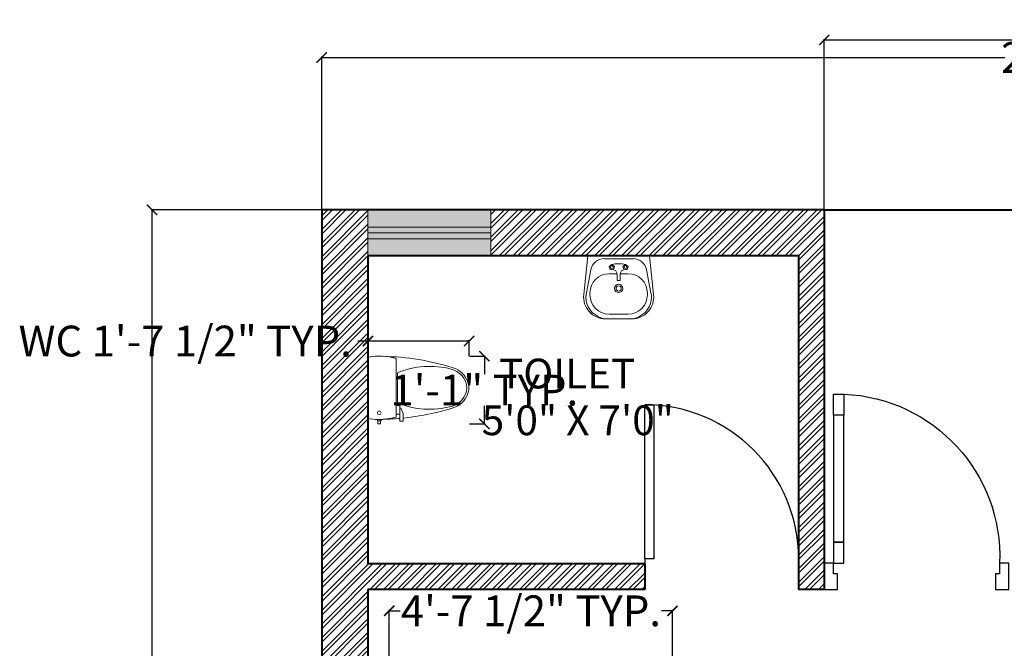
# Model space of a CAD drawing. Units: inches. Extents: x 528 to 2520, y -151 to 1354.
# Tile 7 of 41: x 528 to 720, y 1232 to 1354. Entities that reach past the tile are written whole.
import ezdxf

# ---------------------------------------------------------------- set-up
doc = ezdxf.new("R2010")
doc.units = ezdxf.units.IN
doc.header["$MEASUREMENT"] = 0
for name, color, linetype, lineweight in [('A-ANNO-DIMS', 2, 'Continuous', 18), ('A-AREA-IDEN', 7, 'Continuous', 18), ('A-Door', 150, 'Continuous', 25), ('A-FLOR-FIXT', 9, 'Continuous', 18), ('A-WALL-PATT', 6, 'Continuous', 13), ('walls', 7, 'Continuous', 40), ('WINDOWS', 2, 'Continuous', 20)]:
    doc.layers.add(name, color=color, linetype=linetype, lineweight=lineweight)
doc.layers.add('A-GLAZ-PATT', color=152, linetype='Continuous', lineweight=13, true_color=0x2776bb)
doc.layers.add('NT', color=1, linetype='Continuous')
doc.styles.get("Standard").update_dxf_attribs({"font": 'arial.ttf'})
doc.dimstyles.get("Standard").update_dxf_attribs({"dimtxt": 6, "dimasz": 2, "dimexe": 0.18, "dimexo": 0.0625, "dimgap": 0.09, "dimtad": 0, "dimtih": 1, "dimtoh": 1, "dimdec": 1, "dimzin": 0, "dimdsep": 46, "dimlunit": 3, "dimtxsty": 'Standard', "dimblk": 'ARCHTICK', "dimcen": 0.09, "dimadec": 0, "dimazin": 0, "dimtfac": 1, "dimtdec": 1, "dimtofl": 0, "dimtmove": 0, "dimatfit": 3, "dimfxl": 1, "dimtolj": 1, "dimtzin": 0, "dimarcsym": 0})

# ---------------------------------------------------------------- blocks, each defined once
blk = doc.blocks.new('A$C7DB75F4D')
at = {"layer": 'A-Door'}
for points in [[(625, 740), (625, 660), (665, 660), (665, 740)], [(625, 180), (625, 660), (665, 660), (665, 180)], [(625, 100), (625, 180), (665, 180), (665, 100)], [(35, 100), (35, 60), (50, 60), (50, 50), (50, 0), (0, 0), (0, 100)], [(665, 100), (700, 100), (700, 0), (650, 0), (650, 50), (650, 60), (665, 60)]]:
    blk.add_lwpolyline(points, close=True, dxfattribs=at)
at = {"layer": 'NT'}
blk.add_arc((650, 125), 615.5, 92.3278, 182.3278, dxfattribs=at)
blk = doc.blocks.new('toilet-7')
at = {"color": 0, "linetype": 'ByBlock'}
for p, q in [((0.2097, -0.02), (-0.2097, -0.02)), ((0.2151, -0.0677), (0.2097, -0.02)), ((-0.2457, -0.0874), (-0.2457, -0.1068)), ((-0.2457, -0.0874), (-0.2257, -0.0874)), ((-0.2457, -0.1068), (-0.2257, -0.1068)), ((-0.2257, -0.0846), (-0.2257, -0.1096)), ((-0.2257, -0.0846), (-0.2157, -0.0846)), ((-0.2257, -0.1096), (-0.2154, -0.1096)), ((0.2099, -0.164), (0.2151, -0.1171)), ((0.2151, -0.1171), (0.2151, -0.0677)), ((0.1991, -0.2124), (0.2099, -0.164)), ((-0.1213, -0.2374), (-0.2278, -0.2374)), ((-0.2278, -0.2374), (-0.2278, -0.2599)), ((-0.1759, -0.2599), (-0.2278, -0.2599)), ((0.1991, -0.2124), (-0.1991, -0.2124)), ((-0.1803, -0.2374), (-0.1803, -0.2124)), ((-0.1759, -0.2599), (-0.1379, -0.2451)), ((-0.1379, -0.2451), (-0.1379, -0.2374)), ((-0.1213, -0.2374), (-0.1213, -0.2124)), ((-0.1023, -0.2212), (0.1023, -0.2212))]:
    blk.add_line(p, q, dxfattribs=at)
blk.add_circle((-0.1696, -0.0971), 0.0125, dxfattribs=at)
for centre, radius, start, end in [((0.2244, -0.0924), 0.4402, 170.53768, 187.73995), ((1.517, -0.087), 1.7318, 181.22237, 184.98223), ((-1.517, -0.087), 1.7318, 342.75226, 358.77763), ((0.2244, -0.0924), 0.4402, 187.73995, 195.82198), ((1.517, -0.087), 1.7318, 185.73228, 197.24774), ((0.4258, -0.4413), 0.5721, 157.37374, 194.77857), ((-0.4258, -0.4413), 0.5721, 345.22143, 22.62626), ((0.0116, -0.5544), 0.1554, 197.24774, 249.54761), ((0.0221, -0.5478), 0.1546, 194.77857, 226.85426), ((-0.0116, -0.5544), 0.1554, 290.45239, 342.75226), ((-0.0221, -0.5478), 0.1546, 313.14574, 345.22143), ((0, -0.5713), 0.1223, 226.85426, 313.14574), ((0, -0.5854), 0.1223, 249.54761, 290.45239)]:
    blk.add_arc(centre, radius, start, end, dxfattribs=at)
blk = doc.blocks.new('_ArchTick')
at = {"color": 0, "linetype": 'ByBlock', "const_width": 0.15}
blk.add_lwpolyline([(-0.5, -0.5), (0.5, 0.5)], dxfattribs=at)
blk = doc.blocks.new('*D25')
at = {"layer": 'A-ANNO-DIMS', "color": 0, "lineweight": -2, "transparency": 16777216}
for p, q in [((586.7, 1317.17), (586.7, 1346.96)), ((586.7, 1346.78), (719.92, 1346.78)), ((885.7, 1346.78), (752.47, 1346.78)), ((885.7, 1317.17), (885.7, 1346.96))]:
    blk.add_line(p, q, dxfattribs=at)
at = {"layer": 'Defpoints', "color": 0, "transparency": 16777216}
for p in [(885.7, 1346.78), (586.7, 1317.1), (885.7, 1317.1)]:
    blk.add_point(p, dxfattribs=at)
at = {"layer": 'A-ANNO-DIMS', "color": 0, "lineweight": -2, "transparency": 16777216, "xscale": 2, "yscale": 2, "zscale": 2, "rotation": 180}
blk.add_blockref('_ArchTick', (586.7, 1346.78), dxfattribs=at)
at = {"layer": 'A-ANNO-DIMS', "color": 0, "lineweight": -2, "transparency": 16777216, "xscale": 2, "yscale": 2, "zscale": 2}
blk.add_blockref('_ArchTick', (885.7, 1346.78), dxfattribs=at)
at = {"layer": 'A-ANNO-DIMS', "color": 0, "transparency": 16777216, "insert": (736.2, 1346.78), "char_height": 6, "attachment_point": 5}
blk.add_mtext('\\A1;24\'-11.0"', dxfattribs=at)
blk = doc.blocks.new('BASIN-WITH-TAP')
for p, q in [((0.84, 12.27), (0.02, 4.73)), ((12.84, 12.27), (0.84, 12.27)), ((9.64, 11.73), (4.05, 11.73)), ((12.84, 12.27), (13.66, 4.73)), ((5, 10.24), (5.51, 10.61)), ((5.2, 9.64), (5, 10.24)), ((5.24, 10.1), (5.2, 10.1)), ((5.24, 9.64), (5.51, 9.64)), ((5.51, 10.61), (6.02, 10.24)), ((6.02, 10.24), (5.82, 9.64)), ((8.18, 10.61), (7.67, 10.24)), ((7.67, 10.24), (7.86, 9.64)), ((8.68, 10.24), (8.18, 10.61)), ((8.49, 9.64), (8.18, 9.64)), ((8.44, 10.1), (8.49, 10.1)), ((8.49, 9.64), (8.68, 10.24)), ((1.43, 9.58), (0.55, 5.09)), ((4.98, 8.8), (6.58, 8.8)), ((6.58, 8.31), (6.58, 8.58)), ((6.58, 7.51), (6.58, 8.31)), ((8.71, 8.8), (7.11, 8.8)), ((7.11, 8.31), (7.11, 8.58)), ((7.11, 7.51), (7.11, 8.31)), ((12.26, 9.58), (13.14, 5.09)), ((6.58, 7.51), (7.11, 7.51)), ((1.24, 4.67), (1.24, 5.07)), ((12.44, 4.67), (12.44, 5.07)), ((4.73, 0), (8.96, 0)), ((6.84, 0.93), (4.98, 0.93)), ((6.84, 0.93), (8.71, 0.93))]:
    blk.add_line(p, q)
for centre, radius in [((5.5, 10.1), 0.277), ((8.19, 10.1), 0.277), ((6.84, 5.94), 0.821), ((6.84, 5.94), 0.507)]:
    blk.add_circle(centre, radius)
for centre, radius, start, end in [((4.05, 9.07), 2.67, 90, 168.8773), ((9.64, 9.07), 2.67, 11.1227, 90), ((6.84, 4.01), 6.73, 78.5788, 101.4212), ((5.51, 8.58), 1.07, 0, 90), ((8.18, 8.58), 1.07, 90, 180), ((4.98, 5.07), 3.73, 90, 180), ((8.71, 5.07), 3.73, 0, 90), ((4.27, 4.27), 4.27, 173.7966, 270), ((4.73, 4.27), 4.27, 168.8773, 270), ((4.98, 4.67), 3.73, 180, 270), ((8.71, 4.67), 3.73, 270, 0), ((8.96, 4.27), 4.27, 270, 11.1227), ((9.42, 4.27), 4.27, 270, 6.2034)]:
    blk.add_arc(centre, radius, start, end)
blk = doc.blocks.new('DOOR-SWING-30')
for p, q in [((0, 6), (0, 0)), ((30, 6), (30, 0))]:
    blk.add_line(p, q)
blk.add_lwpolyline([(0, 6), (0, 36), (1.75, 36), (1.75, 6)], close=True)
blk.add_arc((0, 6), 30, 0, 90)
blk = doc.blocks.new('WINDOW-24x9-PLAN')
for p, q in [((0, 5.63), (24, 5.63)), ((0, 4.5), (24, 4.5)), ((0, 3.37), (24, 3.37))]:
    blk.add_line(p, q)
blk.add_lwpolyline([(0, 9), (24, 9), (24, 0), (0, 0)], close=True)
blk = doc.blocks.new('*D47')
at = {"layer": 'A-ANNO-DIMS', "color": 0, "lineweight": -2, "transparency": 16777216}
for p, q in [((599.87, 1227.49), (599.87, 1239.13)), ((599.87, 1238.95), (602.01, 1238.95)), ((655.12, 1238.95), (652.98, 1238.95)), ((655.12, 1227.49), (655.12, 1239.13))]:
    blk.add_line(p, q, dxfattribs=at)
at = {"layer": 'Defpoints', "color": 0, "transparency": 16777216}
for p in [(599.87, 1238.95), (599.87, 1227.43), (655.12, 1227.43)]:
    blk.add_point(p, dxfattribs=at)
at = {"layer": 'A-ANNO-DIMS', "color": 0, "lineweight": -2, "transparency": 16777216, "xscale": 2, "yscale": 2, "zscale": 2, "rotation": 180}
blk.add_blockref('_ArchTick', (599.87, 1238.95), dxfattribs=at)
at = {"layer": 'A-ANNO-DIMS', "color": 0, "lineweight": -2, "transparency": 16777216, "xscale": 2, "yscale": 2, "zscale": 2}
blk.add_blockref('_ArchTick', (655.12, 1238.95), dxfattribs=at)
at = {"layer": 'A-ANNO-DIMS', "color": 0, "transparency": 16777216, "insert": (627.5, 1238.95), "char_height": 6, "attachment_point": 5}
blk.add_mtext('\\A1;4\'-7 1/2" TYP.', dxfattribs=at)
blk = doc.blocks.new('*D50')
at = {"layer": 'A-ANNO-DIMS', "color": 0, "lineweight": -2, "transparency": 16777216}
for p, q in [((595.72, 1291.52), (593.72, 1291.52)), ((595.72, 1288.62), (595.72, 1291.7)), ((615.46, 1291.52), (595.72, 1291.52)), ((615.46, 1288.62), (615.46, 1291.7))]:
    blk.add_line(p, q, dxfattribs=at)
at = {"layer": 'Defpoints', "color": 0, "transparency": 16777216}
for p in [(595.72, 1291.52), (595.72, 1288.56), (615.46, 1288.56)]:
    blk.add_point(p, dxfattribs=at)
at = {"layer": 'A-ANNO-DIMS', "color": 0, "lineweight": -2, "transparency": 16777216, "xscale": 2, "yscale": 2, "zscale": 2, "rotation": 180}
blk.add_blockref('_ArchTick', (595.72, 1291.52), dxfattribs=at)
at = {"layer": 'A-ANNO-DIMS', "color": 0, "lineweight": -2, "transparency": 16777216, "xscale": 2, "yscale": 2, "zscale": 2}
blk.add_blockref('_ArchTick', (615.46, 1291.52), dxfattribs=at)
at = {"layer": 'A-ANNO-DIMS', "color": 0, "transparency": 16777216, "insert": (560.08, 1291.52), "char_height": 6, "attachment_point": 5}
blk.add_mtext('\\A1;WC 1\'-7 1/2" TYP.', dxfattribs=at)
blk = doc.blocks.new('*D51')
at = {"layer": 'A-ANNO-DIMS', "color": 0, "lineweight": -2, "transparency": 16777216}
for p, q in [((615.52, 1288.56), (618.6, 1288.56)), ((618.42, 1288.56), (618.42, 1285.08)), ((618.42, 1275.38), (618.42, 1278.87)), ((615.52, 1275.38), (618.6, 1275.38))]:
    blk.add_line(p, q, dxfattribs=at)
at = {"layer": 'Defpoints', "color": 0, "transparency": 16777216}
for p in [(615.46, 1288.56), (618.42, 1288.56), (615.46, 1275.38)]:
    blk.add_point(p, dxfattribs=at)
at = {"layer": 'A-ANNO-DIMS', "color": 0, "lineweight": -2, "transparency": 16777216, "xscale": 2, "yscale": 2, "zscale": 2}
for p, rotation in [((618.42, 1288.56), 90), ((618.42, 1275.38), 270)]:
    blk.add_blockref('_ArchTick', p, dxfattribs=dict(at, rotation=rotation))
at = {"layer": 'A-ANNO-DIMS', "color": 0, "transparency": 16777216, "insert": (618.42, 1281.97), "char_height": 6, "attachment_point": 5}
blk.add_mtext('\\A1;1\'-1" TYP.', dxfattribs=at)
blk = doc.blocks.new('*D92')
at = {"layer": 'A-ANNO-DIMS', "color": 0, "lineweight": -2, "transparency": 16777216}
for p, q in [((586.63, 1317.1), (553.42, 1317.1)), ((553.6, 1317.1), (553.6, 1051.76)), ((553.6, 780.1), (553.6, 1045.45)), ((586.63, 780.1), (553.42, 780.1))]:
    blk.add_line(p, q, dxfattribs=at)
at = {"layer": 'Defpoints', "color": 0, "transparency": 16777216}
for p in [(553.6, 1317.1), (586.7, 1317.1), (586.7, 780.1)]:
    blk.add_point(p, dxfattribs=at)
at = {"layer": 'A-ANNO-DIMS', "color": 0, "lineweight": -2, "transparency": 16777216, "xscale": 2, "yscale": 2, "zscale": 2}
for p, rotation in [((553.6, 1317.1), 90), ((553.6, 780.1), 270)]:
    blk.add_blockref('_ArchTick', p, dxfattribs=dict(at, rotation=rotation))
at = {"layer": 'A-ANNO-DIMS', "color": 0, "transparency": 16777216, "insert": (553.6, 1048.6), "char_height": 6, "attachment_point": 5}
blk.add_mtext('\\A1;44\'-9"', dxfattribs=at)
blk = doc.blocks.new('*D93')
at = {"layer": 'A-ANNO-DIMS', "color": 0, "lineweight": -2, "transparency": 16777216}
for p, q in [((684.7, 1317.17), (684.7, 1350.38)), ((684.7, 1350.2), (728.13, 1350.2)), ((787.7, 1350.2), (744.27, 1350.2)), ((787.7, 1317.17), (787.7, 1350.38))]:
    blk.add_line(p, q, dxfattribs=at)
at = {"layer": 'Defpoints', "color": 0, "transparency": 16777216}
for p in [(787.7, 1350.2), (684.7, 1317.1), (787.7, 1317.1)]:
    blk.add_point(p, dxfattribs=at)
at = {"layer": 'A-ANNO-DIMS', "color": 0, "lineweight": -2, "transparency": 16777216, "xscale": 2, "yscale": 2, "zscale": 2, "rotation": 180}
blk.add_blockref('_ArchTick', (684.7, 1350.2), dxfattribs=at)
at = {"layer": 'A-ANNO-DIMS', "color": 0, "lineweight": -2, "transparency": 16777216, "xscale": 2, "yscale": 2, "zscale": 2}
blk.add_blockref('_ArchTick', (787.7, 1350.2), dxfattribs=at)
at = {"layer": 'A-ANNO-DIMS', "color": 0, "transparency": 16777216, "insert": (736.2, 1350.2), "char_height": 6, "attachment_point": 5}
blk.add_mtext('\\A1;8\'-7"', dxfattribs=at)

msp = doc.modelspace()

# ---------------------------------------------------------------- hatches: boundary and pattern name
at = {"layer": 'A-GLAZ-PATT'}
h = msp.add_hatch(color=256, dxfattribs=at)
h.dxf.hatch_style = 1
h.paths.add_polyline_path([(619.7, 1313.73), (595.7, 1313.73), (595.7, 1312.6), (619.7, 1312.6)])
h.paths.add_polyline_path([(619.7, 1312.6), (595.7, 1312.6), (595.7, 1311.47), (619.7, 1311.47)])
h.paths.add_polyline_path([(619.7, 1317.1), (595.7, 1317.1), (595.7, 1313.73), (619.7, 1313.73)])
h.paths.add_polyline_path([(619.7, 1311.47), (595.7, 1311.47), (595.7, 1308.1), (619.7, 1308.1)])
at = {"layer": 'A-WALL-PATT'}
h = msp.add_hatch(dxfattribs=at)
h.set_pattern_fill('ANSI32', color=256, scale=5)
h.paths.add_polyline_path([(595.7, 1163.86), (586.7, 1163.86), (586.7, 969.1), (598.24, 969.1), (603.24, 969.1), (603.24, 974.1), (595.7, 974.1), (595.7, 1082.1), (691.7, 1082.1), (691.7, 1087.1), (691.7, 1106.1), (697.7, 1106.1), (697.7, 1111.1), (686.7, 1111.1), (686.7, 1087.1), (595.7, 1087.1)])
h.paths.add_polyline_path([(688.7, 974.1), (651.24, 974.1), (651.24, 969.1), (688.7, 969.1)])
h.paths.add_polyline_path([(885.7, 1171.37), (876.7, 1171.37), (876.7, 1111.1), (786.7, 1111.1), (786.7, 1106.1), (876.7, 1106.1), (876.7, 974.1), (786.7, 974.1), (786.7, 969.1), (876.7, 969.1), (876.7, 825.1), (834.7, 825.1), (834.7, 816.1), (885.7, 816.1)])
h.paths.add_polyline_path([(885.7, 1317.1), (876.65, 1317.1), (876.65, 1308.1), (876.7, 1308.1), (876.7, 1248.1), (822.7, 1248.1), (822.7, 1243.1), (876.7, 1243.1), (876.7, 1219.37), (885.7, 1219.37)])
h.paths.add_polyline_path([(852.65, 1317.1), (787.7, 1317.1), (787.7, 1248.1), (784.26, 1248.1), (784.26, 1243.1), (792.7, 1243.1), (792.7, 1249.1), (792.7, 1308.1), (852.65, 1308.1)])
h.paths.add_polyline_path([(684.7, 1317.1), (619.7, 1317.1), (619.7, 1308.1), (679.7, 1308.1), (679.7, 1248.1), (679.7, 1243.1), (684.7, 1243.1), (684.7, 1248.25)])
h.paths.add_polyline_path([(595.7, 1308.1), (595.7, 1317.1), (586.7, 1317.1), (586.7, 1211.86), (595.7, 1211.86), (595.7, 1243.1), (649.7, 1243.1), (649.7, 1248.1), (595.7, 1248.1)])
h.paths.add_polyline_path([(744.7, 969.1), (744.7, 974.1), (724.7, 974.1), (724.7, 969.1), (739.7, 969.1), (739.7, 874.29), (744.7, 874.29)])
h.paths.add_polyline_path([(739.7, 969.1), (727.7, 969.1), (727.7, 965.12), (730.74, 965.12), (730.74, 961.68), (734.43, 961.68), (734.43, 957.24), (739.7, 957.24)], flags=17)
h.paths.add_polyline_path([(786.7, 825.1), (744.7, 825.1), (744.7, 832.29), (739.7, 832.29), (739.7, 816.1), (786.7, 816.1)])

# ---------------------------------------------------------------- linework, layer by layer
at = {"layer": 'walls'}
for p, q in [((586.7, 1317.1), (586.7, 789.1)), ((684.7, 1317.1), (586.7, 1317.1)), ((684.7, 1317.1), (684.7, 1248.1)), ((684.7, 1317.1), (787.7, 1317.1)), ((595.7, 1308.1), (595.7, 1248.1)), ((679.7, 1308.1), (595.7, 1308.1)), ((679.7, 1308.1), (679.7, 1248.1)), ((649.7, 1248.1), (595.7, 1248.1)), ((649.7, 1248.1), (649.7, 1243.1)), ((679.7, 1248.1), (679.7, 1243.1)), ((684.7, 1248.1), (684.7, 1243.1)), ((595.7, 1243.1), (595.7, 1087.1)), ((649.7, 1243.1), (595.7, 1243.1)), ((684.7, 1243.1), (679.7, 1243.1))]:
    msp.add_line(p, q, dxfattribs=at)

# ---------------------------------------------------------------- block references
at = {"layer": 'A-Door', "xscale": -0.0514539602427209, "yscale": 0.0514539602427209, "zscale": 0.0514539602427209}
msp.add_blockref('A$C7DB75F4D', (720.71, 1243.1), dxfattribs=at)
at = {"layer": 'A-Door'}
msp.add_blockref('DOOR-SWING-30', (649.7, 1243.1), dxfattribs=at)
at = {"layer": 'A-FLOR-FIXT'}
msp.add_blockref('BASIN-WITH-TAP', (637.77, 1295.84), dxfattribs=at)
at = {"layer": 'A-FLOR-FIXT', "xscale": 28.60654769571749, "yscale": 28.60654769571749, "zscale": 28.60654769571749, "rotation": 90}
msp.add_blockref('toilet-7', (595.14, 1282.41), dxfattribs=at)
at = {"layer": 'WINDOWS'}
msp.add_blockref('WINDOW-24x9-PLAN', (595.7, 1308.1), dxfattribs=at)

# ---------------------------------------------------------------- texts
at = {"layer": 'A-AREA-IDEN'}
for s, height, p in [('TOILET', 5.793, (621.27, 1282.29)), ('5\'0" X 7\'0"', 5.7926, (617.9, 1273.18))]:
    msp.add_text(s, height=height, dxfattribs=at).set_placement(p)

# ---------------------------------------------------------------- dimensions: what is measured, and where the dimension line sits
at = {"layer": 'A-ANNO-DIMS'}
for base, p1, p2, override, picture, middle in [((787.7, 1350.2), (684.7, 1317.1), (787.7, 1317.1), {"dimdec": 1, "dimlfac": 1, "dimrnd": 0, "dimzin": 1, "dimdsep": 46, "dimlunit": 4, "dimfrac": 2}, '*D93', (736.2, 1350.2)), ((885.7, 1346.78), (586.7, 1317.1), (885.7, 1317.1), {"dimclrd": 0, "dimclre": 0, "dimclrt": 0}, '*D25', (736.2, 1346.78))]:
    dim = msp.add_linear_dim(base=base, p1=p1, p2=p2, dimstyle='Standard', override=override, dxfattribs=at)
    dim.commit()
    dim.dimension.update_dxf_attribs({"geometry": picture, "text_midpoint": middle})
dim = msp.add_linear_dim(base=(553.6, 1317.1), p1=(586.7, 780.1), p2=(586.7, 1317.1), angle=90, dimstyle='Standard', override={"dimdec": 1, "dimlfac": 1, "dimrnd": 0, "dimzin": 1, "dimdsep": 46, "dimlunit": 4, "dimfrac": 2}, dxfattribs=at)
dim.commit()
dim.dimension.update_dxf_attribs({"geometry": '*D92', "text_midpoint": (553.6, 1048.6)})
for base, p1, p2, angle, text, picture, middle in [((595.72, 1291.52), (615.46, 1288.56), (595.72, 1288.56), 180, 'WC <> TYP.', '*D50', (560.08, 1291.52)), ((618.42, 1288.56), (615.46, 1275.38), (615.46, 1288.56), 90, '<> TYP.', '*D51', (618.42, 1281.97)), ((599.8695, 1238.951), (655.1213, 1227.431), (599.8695, 1227.431), 180, '<> TYP.', '*D47', (627.4954, 1238.951))]:
    dim = msp.add_linear_dim(base=base, p1=p1, p2=p2, angle=angle, text=text, dimstyle='Standard', override={"dimdec": 1, "dimlfac": 1, "dimrnd": 0, "dimzin": 1, "dimdsep": 46, "dimlunit": 4, "dimfrac": 2}, dxfattribs=at)
    dim.commit()
    dim.dimension.update_dxf_attribs({"geometry": picture, "text_midpoint": middle})

doc.saveas('drawing.dxf')
